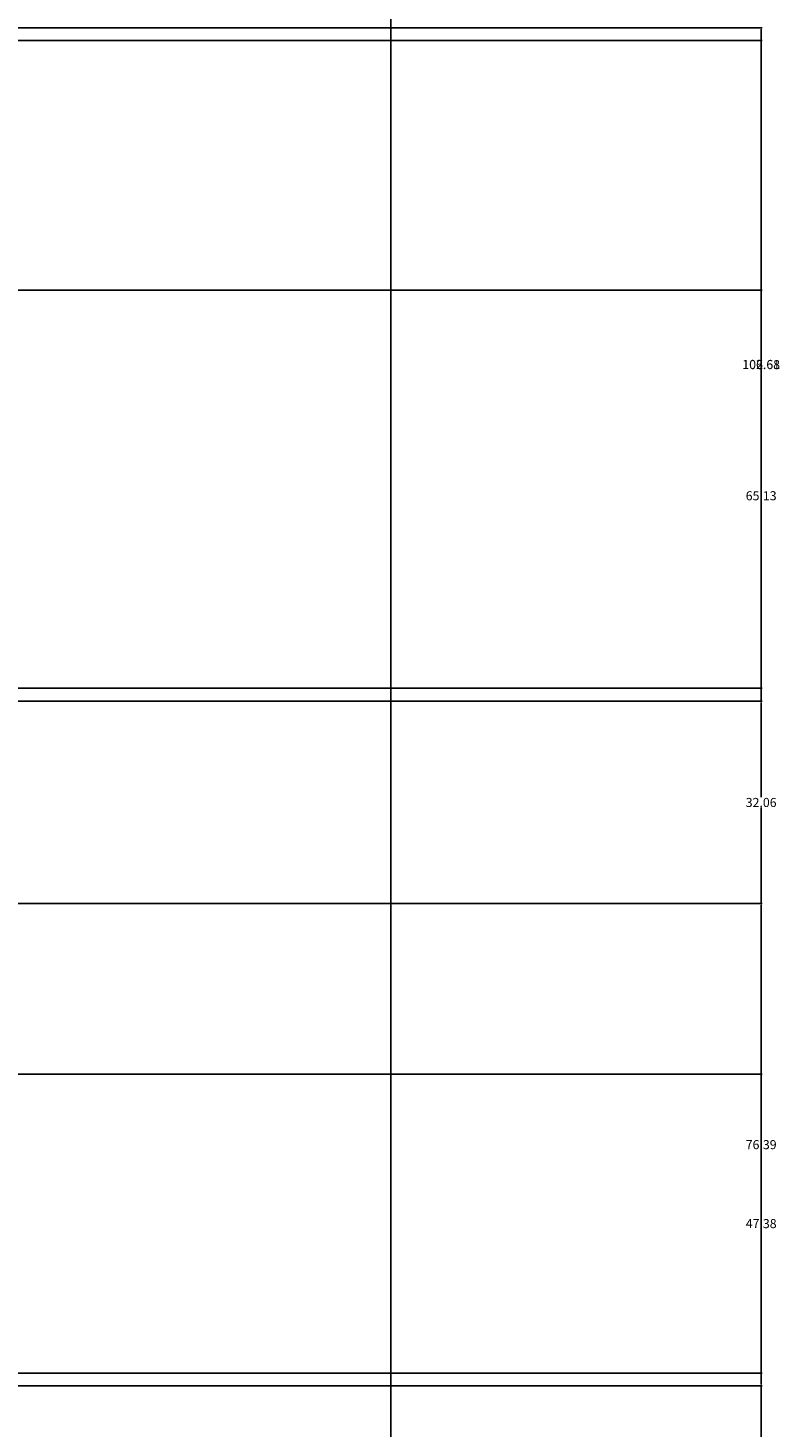
# Model space of a CAD drawing. Units: inches. Extents: x 241 to 943, y 109 to 1396.
# Tile 17 of 34: x 824 to 943, y 620 to 842. Entities that reach past the tile are written whole.
import ezdxf

# ---------------------------------------------------------------- set-up
doc = ezdxf.new("R2010")
doc.units = ezdxf.units.IN
doc.header["$MEASUREMENT"] = 0
doc.layers.add('A-ANNO-DIMS', color=2, linetype='Continuous', lineweight=18)
doc.styles.get("Standard").update_dxf_attribs({"font": 'arial.ttf'})
doc.dimstyles.get("Standard").update_dxf_attribs({"dimtxt": 1.4375, "dimasz": 0.18, "dimexe": 0.18, "dimexo": 0.0625, "dimgap": 0.09, "dimtad": 0, "dimtih": 1, "dimtoh": 1, "dimdec": 4, "dimzin": 0, "dimdsep": 46, "dimlunit": 4, "dimtxsty": 'Standard', "dimcen": 0.09, "dimadec": 0, "dimazin": 0, "dimtfac": 1, "dimtdec": 4, "dimtofl": 0, "dimtmove": 0, "dimatfit": 3, "dimfxl": 1, "dimtolj": 1, "dimtzin": 0, "dimarcsym": 0})

# ---------------------------------------------------------------- blocks, each defined once
blk = doc.blocks.new('*D6')
at = {"layer": 'A-ANNO-DIMS', "color": 0, "lineweight": -2, "transparency": 16777216}
for p, q in [((820.84, 232.89), (820.84, 1395.05)), ((821.02, 1394.87), (848.73, 1394.87)), ((881.49, 1394.87), (853.77, 1394.87)), ((881.67, 232.89), (881.67, 1395.05))]:
    blk.add_line(p, q, dxfattribs=at)
at = {"layer": 'A-ANNO-DIMS', "color": 0, "transparency": 16777216}
for points in [[(821.02, 1394.9), (821.02, 1394.84), (820.84, 1394.87)], [(881.49, 1394.9), (881.49, 1394.84), (881.67, 1394.87)]]:
    blk.add_solid(points, dxfattribs=at)
at = {"layer": 'Defpoints', "color": 0, "transparency": 16777216}
for p in [(881.67, 1394.87), (820.84, 232.83), (881.67, 232.83)]:
    blk.add_point(p, dxfattribs=at)
at = {"layer": 'A-ANNO-DIMS', "color": 0, "transparency": 16777216, "insert": (851.25, 1394.87), "char_height": 1.438, "attachment_point": 5}
blk.add_mtext('\\A1;60.83', dxfattribs=at)
blk = doc.blocks.new('*D46')
at = {"layer": 'A-ANNO-DIMS', "color": 0, "lineweight": -2, "transparency": 16777216}
for p, q in [((749.7, 702.79), (940.6, 702.79)), ((940.42, 702.61), (940.42, 665.42)), ((940.42, 626.58), (940.42, 663.77)), ((749.7, 626.4), (940.6, 626.4))]:
    blk.add_line(p, q, dxfattribs=at)
at = {"layer": 'A-ANNO-DIMS', "color": 0, "transparency": 16777216}
for points in [[(940.39, 702.61), (940.45, 702.61), (940.42, 702.79)], [(940.39, 626.58), (940.45, 626.58), (940.42, 626.4)]]:
    blk.add_solid(points, dxfattribs=at)
at = {"layer": 'Defpoints', "color": 0, "transparency": 16777216}
for p in [(749.63, 702.79), (940.42, 702.79), (749.63, 626.4)]:
    blk.add_point(p, dxfattribs=at)
at = {"layer": 'A-ANNO-DIMS', "color": 0, "transparency": 16777216, "insert": (940.42, 664.6), "char_height": 1.438, "attachment_point": 5}
blk.add_mtext('\\A1;76.39', dxfattribs=at)
blk = doc.blocks.new('*D47')
at = {"layer": 'A-ANNO-DIMS', "color": 0, "lineweight": -2, "transparency": 16777216}
for p, q in [((792.75, 841.54), (940.6, 841.54)), ((940.42, 841.36), (940.42, 789.02)), ((940.42, 735.03), (940.42, 787.37)), ((792.75, 734.85), (940.6, 734.85))]:
    blk.add_line(p, q, dxfattribs=at)
at = {"layer": 'A-ANNO-DIMS', "color": 0, "transparency": 16777216}
for points in [[(940.39, 841.36), (940.45, 841.36), (940.42, 841.54)], [(940.39, 735.03), (940.45, 735.03), (940.42, 734.85)]]:
    blk.add_solid(points, dxfattribs=at)
at = {"layer": 'Defpoints', "color": 0, "transparency": 16777216}
for p in [(792.69, 841.54), (940.42, 841.54), (792.69, 734.85)]:
    blk.add_point(p, dxfattribs=at)
at = {"layer": 'A-ANNO-DIMS', "color": 0, "transparency": 16777216, "insert": (940.42, 788.2), "char_height": 1.438, "attachment_point": 5}
blk.add_mtext('\\A1;106.68', dxfattribs=at)
blk = doc.blocks.new('*D85')
at = {"layer": 'A-ANNO-DIMS', "color": 0, "lineweight": -2, "transparency": 16777216}
for p, q in [((749.7, 626.4), (940.6, 626.4)), ((940.42, 626.22), (940.42, 598.44)), ((940.42, 569.01), (940.42, 596.79)), ((792.75, 568.83), (940.6, 568.83))]:
    blk.add_line(p, q, dxfattribs=at)
at = {"layer": 'A-ANNO-DIMS', "color": 0, "transparency": 16777216}
for points in [[(940.39, 626.22), (940.45, 626.22), (940.42, 626.4)], [(940.39, 569.01), (940.45, 569.01), (940.42, 568.83)]]:
    blk.add_solid(points, dxfattribs=at)
at = {"layer": 'Defpoints', "color": 0, "transparency": 16777216}
for p in [(749.63, 626.4), (940.42, 626.4), (792.69, 568.83)]:
    blk.add_point(p, dxfattribs=at)
at = {"layer": 'A-ANNO-DIMS', "color": 0, "transparency": 16777216, "insert": (940.42, 597.62), "char_height": 1.438, "attachment_point": 5}
blk.add_mtext('\\A1;57.57', dxfattribs=at)
blk = doc.blocks.new('*D86')
at = {"layer": 'A-ANNO-DIMS', "color": 0, "lineweight": -2, "transparency": 16777216}
for p, q in [((792.75, 734.85), (940.6, 734.85)), ((940.42, 734.67), (940.42, 719.65)), ((940.42, 702.97), (940.42, 718)), ((749.7, 702.79), (940.6, 702.79))]:
    blk.add_line(p, q, dxfattribs=at)
at = {"layer": 'A-ANNO-DIMS', "color": 0, "transparency": 16777216}
for points in [[(940.39, 734.67), (940.45, 734.67), (940.42, 734.85)], [(940.39, 702.97), (940.45, 702.97), (940.42, 702.79)]]:
    blk.add_solid(points, dxfattribs=at)
at = {"layer": 'Defpoints', "color": 0, "transparency": 16777216}
for p in [(792.69, 734.85), (940.42, 734.85), (749.63, 702.79)]:
    blk.add_point(p, dxfattribs=at)
at = {"layer": 'A-ANNO-DIMS', "color": 0, "transparency": 16777216, "insert": (940.42, 718.82), "char_height": 1.438, "attachment_point": 5}
blk.add_mtext('\\A1;32.06', dxfattribs=at)
blk = doc.blocks.new('*D124')
at = {"layer": 'A-ANNO-DIMS', "color": 0, "lineweight": -2, "transparency": 16777216}
for p, q in [((682.52, 839.54), (940.6, 839.54)), ((940.42, 839.36), (940.42, 789.05)), ((940.42, 737.1), (940.42, 787.41)), ((690.27, 736.92), (940.6, 736.92))]:
    blk.add_line(p, q, dxfattribs=at)
at = {"layer": 'A-ANNO-DIMS', "color": 0, "transparency": 16777216}
for points in [[(940.39, 839.36), (940.45, 839.36), (940.42, 839.54)], [(940.39, 737.1), (940.45, 737.1), (940.42, 736.92)]]:
    blk.add_solid(points, dxfattribs=at)
at = {"layer": 'Defpoints', "color": 0, "transparency": 16777216}
for p in [(682.45, 839.54), (940.42, 839.54), (690.2, 736.92)]:
    blk.add_point(p, dxfattribs=at)
at = {"layer": 'A-ANNO-DIMS', "color": 0, "transparency": 16777216, "insert": (940.42, 788.23), "char_height": 1.438, "attachment_point": 5}
blk.add_mtext('\\A1;102.61', dxfattribs=at)
blk = doc.blocks.new('*D125')
at = {"layer": 'A-ANNO-DIMS', "color": 0, "lineweight": -2, "transparency": 16777216}
for p, q in [((754.6, 799.98), (940.6, 799.98)), ((940.42, 799.8), (940.42, 768.24)), ((940.42, 735.03), (940.42, 766.59)), ((759.69, 734.85), (940.6, 734.85))]:
    blk.add_line(p, q, dxfattribs=at)
at = {"layer": 'A-ANNO-DIMS', "color": 0, "transparency": 16777216}
for points in [[(940.39, 799.8), (940.45, 799.8), (940.42, 799.98)], [(940.39, 735.03), (940.45, 735.03), (940.42, 734.85)]]:
    blk.add_solid(points, dxfattribs=at)
at = {"layer": 'Defpoints', "color": 0, "transparency": 16777216}
for p in [(754.54, 799.98), (940.42, 799.98), (759.62, 734.85)]:
    blk.add_point(p, dxfattribs=at)
at = {"layer": 'A-ANNO-DIMS', "color": 0, "transparency": 16777216, "insert": (940.42, 767.42), "char_height": 1.438, "attachment_point": 5}
blk.add_mtext('\\A1;65.13', dxfattribs=at)
blk = doc.blocks.new('*D135')
at = {"layer": 'A-ANNO-DIMS', "color": 0, "lineweight": -2, "transparency": 16777216}
for p, q in [((678.93, 675.79), (940.6, 675.79)), ((940.42, 675.61), (940.42, 652.92)), ((940.42, 628.58), (940.42, 651.27)), ((678.93, 628.4), (940.6, 628.4))]:
    blk.add_line(p, q, dxfattribs=at)
at = {"layer": 'A-ANNO-DIMS', "color": 0, "transparency": 16777216}
for points in [[(940.39, 675.61), (940.45, 675.61), (940.42, 675.79)], [(940.39, 628.58), (940.45, 628.58), (940.42, 628.4)]]:
    blk.add_solid(points, dxfattribs=at)
at = {"layer": 'Defpoints', "color": 0, "transparency": 16777216}
for p in [(678.87, 675.79), (940.42, 675.79), (678.87, 628.4)]:
    blk.add_point(p, dxfattribs=at)
at = {"layer": 'A-ANNO-DIMS', "color": 0, "transparency": 16777216, "insert": (940.42, 652.09), "char_height": 1.438, "attachment_point": 5}
blk.add_mtext('\\A1;47.38', dxfattribs=at)

msp = doc.modelspace()

# ---------------------------------------------------------------- dimensions: what is measured, and where the dimension line sits
at = {"layer": 'A-ANNO-DIMS'}
dim = msp.add_linear_dim(base=(881.667, 1394.8654), p1=(820.8374, 232.8295), p2=(881.667, 232.8295), dimstyle='Standard', override={"dimdec": 2, "dimlfac": 1, "dimrnd": 0, "dimzin": 0, "dimdsep": 46, "dimlunit": 2}, dxfattribs=at)
dim.commit()
dim.dimension.update_dxf_attribs({"geometry": '*D6', "text_midpoint": (851.2522, 1394.8654)})
for base, p1, p2, picture, middle in [((940.417, 841.5382), (792.691, 734.8538), (792.691, 841.5382), '*D47', (940.417, 788.196)), ((940.417, 839.5382), (690.2047, 736.9235), (682.4526, 839.5382), '*D124', (940.417, 788.2308)), ((940.417, 799.9791), (759.6248, 734.8538), (754.5373, 799.9791), '*D125', (940.417, 767.4165)), ((940.417, 734.8538), (749.6328, 702.7912), (792.691, 734.8538), '*D86', (940.417, 718.8225)), ((940.417, 702.7912), (749.6328, 626.4013), (749.6328, 702.7912), '*D46', (940.417, 664.5962)), ((940.417, 675.7856), (678.8698, 628.4013), (678.8698, 675.7856), '*D135', (940.417, 652.0934)), ((940.417, 626.4013), (792.691, 568.8295), (749.6328, 626.4013), '*D85', (940.417, 597.6154))]:
    dim = msp.add_linear_dim(base=base, p1=p1, p2=p2, angle=90, dimstyle='Standard', override={"dimdec": 2, "dimlfac": 1, "dimrnd": 0, "dimzin": 0, "dimdsep": 46, "dimlunit": 2}, dxfattribs=at)
    dim.commit()
    dim.dimension.update_dxf_attribs({"geometry": picture, "text_midpoint": middle})

doc.saveas('drawing.dxf')
